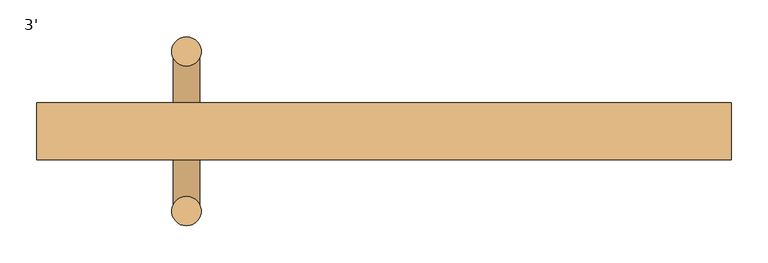
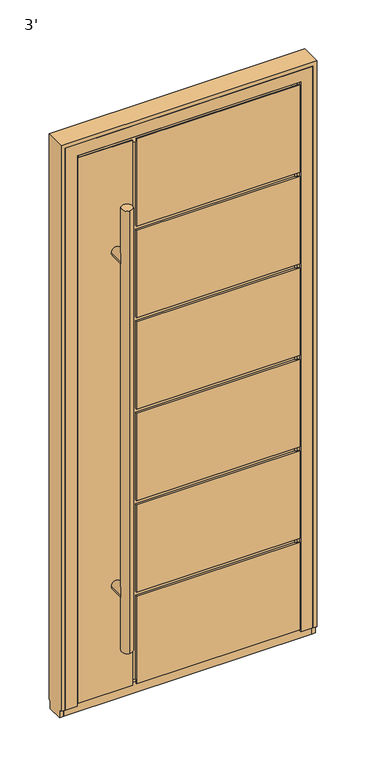
"""IFC4 building model written with IfcOpenShell, lengths in millimetres: door geometry, 3'."""

from ifc_helpers import new_model, si_unit, point, frame, frame_2d, origin, place, context, project, spatial, circle_curve, trimmed, segment, composite_curve, outline, extrude, faceted_brep, source, transform, mapped, element, save


def door_3_79df91aa(model_context):
    return source(origin(), model_context, "Body", "SolidModel", [
        extrude(outline(composite_curve([segment(trimmed(circle_curve(frame_2d((-268.65, 90.8003001)), 20.0), [point((-268.65, 70.8003001))], [point((-268.65, 110.8003001))], False, "CARTESIAN"), True, "CONTINUOUS"), segment(trimmed(circle_curve(frame_2d((-268.65, 90.8003001)), 20.0), [point((-268.65, 110.8003001))], [point((-268.65, 70.8003001))], False, "CARTESIAN"), True, "CONTINUOUS")], self_intersect=False)), frame((0.0, 0.0, 210.0000003), z_axis=(0.0, 0.0, 1.0), x_axis=(1.0, 0.0, 0.0)), (0.0, 0.0, 1.0), 1724.5),
        extrude(outline(composite_curve([segment(trimmed(circle_curve(frame_2d((-268.65, -126.2003001)), 20.0), [point((-268.65, -146.2003001))], [point((-268.65, -106.2003001))], False, "CARTESIAN"), True, "CONTINUOUS"), segment(trimmed(circle_curve(frame_2d((-268.65, -126.2003001)), 20.0), [point((-268.65, -106.2003001))], [point((-268.65, -146.2003001))], False, "CARTESIAN"), True, "CONTINUOUS")], self_intersect=False)), frame((0.0, 0.0, 210.0000003), z_axis=(0.0, 0.0, 1.0), x_axis=(1.0, 0.0, 0.0)), (0.0, 0.0, 1.0), 1724.5),
        extrude(outline(composite_curve([segment(trimmed(circle_curve(frame_2d((422.2500003, -268.65)), 18.0), [point((422.2500003, -286.65))], [point((422.2500003, -250.65))], False, "CARTESIAN"), True, "CONTINUOUS"), segment(trimmed(circle_curve(frame_2d((422.2500003, -268.65)), 18.0), [point((422.2500003, -250.65))], [point((422.2500003, -286.65))], False, "CARTESIAN"), True, "CONTINUOUS")], self_intersect=False)), frame((0.0, -126.2, 0.0), z_axis=(0.0, 1.0, 0.0), x_axis=(0.0, 0.0, 1.0)), (0.0, 0.0, 1.0), 217.0),
        extrude(outline(composite_curve([segment(trimmed(circle_curve(frame_2d((1722.2500003, -268.65)), 18.0), [point((1722.2500003, -286.65))], [point((1722.2500003, -250.65))], False, "CARTESIAN"), True, "CONTINUOUS"), segment(trimmed(circle_curve(frame_2d((1722.2500003, -268.65)), 18.0), [point((1722.2500003, -250.65))], [point((1722.2500003, -286.65))], False, "CARTESIAN"), True, "CONTINUOUS")], self_intersect=False)), frame((0.0, -126.2, 0.0), z_axis=(0.0, 1.0, 0.0), x_axis=(0.0, 0.0, 1.0)), (0.0, 0.0, 1.0), 217.0),
        faceted_brep([(-193.65, 13.8, 366.5833337), (383.65, 13.8, 366.5833337), (383.65, 13.8, 351.5833337), (-193.65, 13.8, 351.5833337), (-193.65, 13.8, 35.0), (-208.65, 13.8, 35.0), (-208.65, 13.8, 2109.5000003), (-193.65, 13.8, 2109.5000003), (-193.65, 13.8, 1792.916667), (383.65, 13.8, 1792.916667), (383.65, 13.8, 1777.916667), (-193.65, 13.8, 1777.916667), (-193.65, 13.8, 1436.3333337), (383.65, 13.8, 1436.3333337), (383.65, 13.8, 1421.3333337), (-193.65, 13.8, 1421.3333337), (-193.65, 13.8, 1079.7500004), (383.65, 13.8, 1079.7500004), (383.65, 13.8, 1064.7500004), (-193.65, 13.8, 1064.7500004), (-193.65, 13.8, 723.166667), (383.65, 13.8, 723.166667), (383.65, 13.8, 708.166667), (-193.65, 13.8, 708.166667), (-193.65, 20.8, 708.166667), (-193.65, 20.8, 366.5833337), (383.65, 20.8, 708.166667), (383.65, 11.7997698, 2109.5000003), (383.65, 11.7997698, 35.0), (383.65, 18.8020472, 35.0), (383.65, 18.8020472, 24.0), (383.65, 20.8, 24.0), (383.65, 20.8, 351.5833337), (383.65, 20.8, 366.5833337), (383.65, 20.8, 723.166667), (383.65, 20.8, 1064.7500004), (383.65, 20.8, 1079.7500004), (383.65, 20.8, 1421.3333337), (383.65, 20.8, 1436.3333337), (383.65, 20.8, 1777.916667), (383.65, 20.8, 1792.916667), (383.65, 20.8, 2109.5000003), (-193.65, 20.8, 723.166667), (-193.65, 20.8, 1064.7500004), (-193.65, 20.8, 1079.7500004), (-193.65, 20.8, 1421.3333337), (-208.65, 18.8020472, 35.0), (-208.65, 18.8020472, 24.0), (-208.65, 20.8, 24.0), (-208.65, 20.8, 2109.5000003), (-383.65, 11.7997698, 35.0), (-383.65, 18.8020472, 35.0), (-193.65, 18.8020472, 35.0), (-193.65, 20.8, 351.5833337), (-193.65, 20.8, 24.0), (-193.65, 18.8020472, 24.0), (-383.65, 18.8020472, 24.0), (-383.65, 20.8, 24.0), (-383.65, 20.8, 2109.5000003), (-193.65, 20.8, 1436.3333337), (-193.65, 20.8, 1777.916667), (-193.65, 20.8, 1792.916667), (-193.65, 20.8, 2109.5000003), (408.65, -56.2, 10.0000003), (-193.65, -56.2, 10.0000003), (-193.65, -53.2, 10.0000003), (408.65, -53.2, 10.0000003), (-408.65, -53.2, 10.0000003), (-208.65, -53.2, 10.0000003), (-208.65, -56.2, 10.0000003), (-408.65, -56.2, 10.0000003), (408.65, -56.2, 366.5833337), (408.65, -53.2, 366.5833337), (408.65, -53.2, 708.166667), (408.65, -56.2, 708.166667), (408.65, -56.2, 1079.7500004), (408.65, -53.2, 1079.7500004), (408.65, -53.2, 1421.3333337), (408.65, -56.2, 1421.3333337), (408.65, -56.2, 723.166667), (408.65, -53.2, 723.166667), (408.65, -53.2, 1064.7500004), (408.65, -56.2, 1064.7500004), (408.65, -56.2, 1436.3333337), (408.65, -53.2, 1436.3333337), (408.65, -53.2, 1777.916667), (408.65, -56.2, 1777.916667), (408.65, -56.2, 2134.5000003), (408.65, -56.2, 1792.916667), (408.65, -53.2, 1792.916667), (408.65, -53.2, 2134.5000003), (408.65, -53.2, 351.5833337), (408.65, -56.2, 351.5833337), (-193.65, -53.2, 25.5), (393.15, -53.2, 25.5), (393.15, -53.2, 351.5833337), (393.15, -53.2, 366.5833337), (393.15, -53.2, 708.166667), (393.15, -53.2, 1079.7500004), (393.15, -53.2, 1421.3333337), (393.15, -53.2, 723.166667), (393.15, -53.2, 1064.7500004), (-393.15, -53.2, 25.5), (-208.65, -53.2, 25.5), (-408.65, -53.2, 2134.5000003), (-208.65, -53.2, 2134.5000003), (-208.65, -53.2, 2119.0000003), (-393.15, -53.2, 2119.0000003), (393.15, -53.2, 1436.3333337), (393.15, -53.2, 1777.916667), (393.15, -53.2, 1792.916667), (393.15, -53.2, 2119.0000003), (-193.65, -53.2, 2119.0000003), (-193.65, -53.2, 2134.5000003), (-193.65, -49.2, 351.5833337), (-193.65, -49.2, 25.5), (-193.65, -56.2, 351.5833337), (-208.65, -56.2, 2134.5000003), (-408.65, -56.2, 2134.5000003), (-193.65, -56.2, 708.166667), (-193.65, -56.2, 366.5833337), (-193.65, -56.2, 1421.3333337), (-193.65, -56.2, 1079.7500004), (-193.65, -56.2, 1064.7500004), (-193.65, -56.2, 723.166667), (-193.65, -56.2, 1777.916667), (-193.65, -56.2, 1436.3333337), (-193.65, -56.2, 2134.5000003), (-193.65, -56.2, 1792.916667), (-208.65, -49.2, 2119.0000003), (-208.65, -49.2, 25.5), (-383.65, 11.7997698, 2109.5000003), (393.15, 11.7997698, 2119.0000003), (393.15, 11.7997698, 25.5), (-393.15, 11.7997698, 25.5), (-393.15, 11.7997698, 2119.0000003), (393.15, -49.2, 1792.916667), (393.15, -49.2, 1777.916667), (393.15, -49.2, 1436.3333337), (393.15, -49.2, 1421.3333337), (393.15, -49.2, 1079.7500004), (393.15, -49.2, 1064.7500004), (393.15, -49.2, 723.166667), (393.15, -49.2, 708.166667), (393.15, -49.2, 366.5833337), (393.15, -49.2, 351.5833337), (-193.65, -49.2, 1777.916667), (-193.65, -49.2, 1792.916667), (-193.65, -49.2, 2119.0000003), (-193.65, -49.2, 366.5833337), (-193.65, -49.2, 708.166667), (-193.65, -49.2, 723.166667), (-193.65, -49.2, 1064.7500004), (-193.65, -49.2, 1079.7500004), (-193.65, -49.2, 1421.3333337), (-193.65, -49.2, 1436.3333337)], [[[0, 1, 2, 3, 4, 5, 6, 7, 8, 9, 10, 11, 12, 13, 14, 15, 16, 17, 18, 19, 20, 21, 22, 23]], [[23, 24, 25, 0]], [[23, 22, 26, 24]], [[27, 28, 29, 30, 31, 32, 2, 1, 33, 26, 22, 21, 34, 35, 18, 17, 36, 37, 14, 13, 38, 39, 10, 9, 40, 41]], [[42, 34, 21, 20]], [[19, 43, 42, 20]], [[19, 18, 35, 43]], [[44, 36, 17, 16]], [[15, 45, 44, 16]], [[5, 46, 47, 48, 49, 6]], [[28, 50, 51, 46, 5, 4, 52, 29]], [[53, 54, 55, 52, 4, 3]], [[3, 2, 32, 53]], [[25, 33, 1, 0]], [[29, 52, 55, 30]], [[56, 47, 46, 51]], [[30, 55, 54, 31]], [[57, 48, 47, 56]], [[36, 44, 45, 37]], [[34, 42, 43, 35]], [[33, 25, 24, 26]], [[54, 53, 32, 31]], [[58, 49, 48, 57]], [[38, 59, 60, 39]], [[41, 40, 61, 62]], [[63, 64, 65, 66]], [[67, 68, 69, 70]], [[71, 72, 73, 74]], [[75, 76, 77, 78]], [[79, 80, 81, 82]], [[83, 84, 85, 86]], [[87, 88, 89, 90]], [[66, 91, 92, 63]], [[65, 93, 94, 95, 91, 66]], [[72, 96, 97, 73]], [[76, 98, 99, 77]], [[80, 100, 101, 81]], [[102, 103, 68, 67, 104, 105, 106, 107]], [[84, 108, 109, 85]], [[90, 89, 110, 111, 112, 113]], [[114, 115, 93, 65, 64, 116]], [[70, 69, 117, 118]], [[63, 92, 116, 64]], [[74, 119, 120, 71]], [[78, 121, 122, 75]], [[82, 123, 124, 79]], [[86, 125, 126, 83]], [[87, 127, 128, 88]], [[70, 118, 104, 67]], [[129, 106, 105, 117, 69, 68, 103, 130]], [[58, 57, 56, 51, 50, 131]], [[132, 133, 134, 135], [131, 50, 28, 27]], [[111, 110, 136, 137, 109, 108, 138, 139, 99, 98, 140, 141, 101, 100, 142, 143, 97, 96, 144, 145, 95, 94, 133, 132]], [[94, 93, 115, 130, 103, 102, 134, 133]], [[135, 134, 102, 107]], [[146, 137, 136, 147, 148, 129, 130, 115, 114, 145, 144, 149, 150, 143, 142, 151, 152, 141, 140, 153, 154, 139, 138, 155]], [[153, 122, 121, 154]], [[153, 140, 98, 76, 75, 122]], [[123, 82, 81, 101, 141, 152]], [[151, 124, 123, 152]], [[151, 142, 100, 80, 79, 124]], [[119, 74, 73, 97, 143, 150]], [[149, 120, 119, 150]], [[149, 144, 96, 72, 71, 120]], [[116, 92, 91, 95, 145, 114]], [[15, 14, 37, 45]], [[59, 38, 13, 12]], [[11, 60, 59, 12]], [[11, 10, 39, 60]], [[61, 40, 9, 8]], [[8, 7, 62, 61]], [[125, 86, 85, 109, 137, 146]], [[128, 127, 113, 112, 148, 147]], [[121, 78, 77, 99, 139, 154]], [[155, 138, 108, 84, 83, 126]], [[155, 126, 125, 146]], [[147, 136, 110, 89, 88, 128]], [[90, 113, 127, 87]], [[118, 117, 105, 104]], [[132, 135, 107, 106, 129, 148, 112, 111]], [[27, 41, 62, 7, 6, 49, 58, 131]]]),
        faceted_brep([(-457.2, -56.2, 0.0), (-457.2, -47.1997571, 0.0), (-412.7, -47.1997571, 0.0), (-412.7, -56.2, 0.0), (-403.2, 16.2999958, 0.0), (-403.2, 11.8, 0.0), (-457.2, 11.8, 0.0), (-457.2, 20.8, 0.0), (-387.7, 20.8, 0.0), (-387.7, 16.2999958, 0.0), (457.2, 20.8, 0.0), (457.2, 11.8, 0.0), (403.2, 11.8, 0.0), (403.2, 16.2999958, 0.0), (387.7, 16.2999958, 0.0), (387.7, 20.8, 0.0), (412.7, -47.1997571, 0.0), (457.2, -47.1997571, 0.0), (457.2, -56.2, 0.0), (412.7, -56.2, 0.0), (-457.2, 11.8, -30.0), (-457.2, -47.1997571, -30.0), (-457.2, -56.2, 2189.5), (-457.2, 20.8, 2189.5), (-412.7, -56.2, 2145.0), (412.7, -56.2, 2145.0), (457.2, -56.2, 2189.5), (457.2, 20.8, 2189.5), (457.2, -47.1997571, -30.0), (457.2, 11.8, -30.0), (387.7, 20.8, 2120.0), (-387.7, 20.8, 2120.0), (-403.2, -47.2, 2135.5), (-403.2, -47.2, 14.5), (-403.2, 11.8, 14.5), (-403.2, 16.2999958, 2135.5), (403.2, 16.2999958, 2135.5), (403.2, -47.2, 2135.5), (403.2, 11.8, 14.5), (403.2, -47.2, 14.5), (-412.7, -47.2, 2145.0), (412.7, -47.2, 2145.0), (-387.7, 16.2999958, 2120.0), (387.7, 16.2999958, 2120.0)], [[[0, 1, 2, 3]], [[4, 5, 6, 7, 8, 9]], [[10, 11, 12, 13, 14, 15]], [[16, 17, 18, 19]], [[7, 6, 20, 21, 1, 0, 22, 23]], [[3, 24, 25, 19, 18, 26, 22, 0]], [[22, 26, 27, 23]], [[18, 17, 28, 29, 11, 10, 27, 26]], [[7, 23, 27, 10, 15, 30, 31, 8]], [[32, 33, 34, 5, 4, 35]], [[35, 36, 37, 32]], [[36, 13, 12, 38, 39, 37]], [[40, 24, 3, 2]], [[16, 41, 40, 2, 1, 21, 28, 17], [37, 39, 33, 32]], [[9, 42, 43, 14, 13, 36, 35, 4]], [[8, 31, 42, 9]], [[24, 40, 41, 25]], [[30, 43, 42, 31]], [[19, 25, 41, 16]], [[14, 43, 30, 15]], [[20, 6, 5, 34, 38, 12, 11, 29]], [[39, 38, 34, 33]], [[20, 29, 28, 21]]]),
        faceted_brep([(-457.2, -47.2, -30.0), (-472.2, -47.2, -30.0), (-472.2, 11.8, -30.0), (-457.2, 11.8, -30.0), (-457.2, -56.2, 2189.5), (-457.2, -56.2, 0.0), (-457.2, -47.2, 0.0), (-457.2, 11.8, 0.0), (-457.2, 20.8, 0.0), (-457.2, 20.8, 2189.5), (-472.2, 11.8, 0.0), (472.2, 11.8, 0.0), (472.2, 11.8, -30.0), (457.2, 11.8, -30.0), (457.2, 11.8, 0.0), (-472.2, 20.8, 2204.5), (-472.2, 20.8, 0.0), (-472.2, -47.2, 0.0), (-472.2, -56.2, 0.0), (-472.2, -56.2, 2204.5), (457.2, -47.2, 0.0), (457.2, -47.2, -30.0), (472.2, -47.2, -30.0), (472.2, -47.2, 0.0), (457.2, 20.8, 2189.5), (457.2, 20.8, 0.0), (457.2, -56.2, 0.0), (457.2, -56.2, 2189.5), (472.2, -56.2, 0.0), (472.2, -56.2, 2204.5), (472.2, 20.8, 0.0), (472.2, 20.8, 2204.5)], [[[0, 1, 2, 3]], [[4, 5, 6, 0, 3, 7, 8, 9]], [[7, 3, 2, 10]], [[11, 12, 13, 14]], [[15, 16, 10, 2, 1, 17, 18, 19]], [[17, 1, 0, 6]], [[20, 21, 22, 23]], [[24, 25, 14, 13, 21, 20, 26, 27]], [[27, 26, 28, 29, 19, 18, 5, 4]], [[6, 5, 18, 17]], [[23, 28, 26, 20]], [[22, 21, 13, 12]], [[10, 16, 8, 7]], [[14, 25, 30, 11]], [[9, 8, 16, 15, 31, 30, 25, 24]], [[29, 28, 23, 22, 12, 11, 30, 31]], [[9, 24, 27, 4]], [[19, 29, 31, 15]]]),
    ])


if __name__ == "__main__":
    model = new_model("IFC4")
    model_context = context("Model", 3, world=origin())
    ifc_project = project(units=[si_unit("LENGTHUNIT", "METRE", prefix="MILLI")], contexts=[model_context])
    site = spatial("IfcSite", under=ifc_project)
    building = spatial("IfcBuilding", under=site)
    placement = place(None, origin())
    door_3_shape = door_3_79df91aa(model_context)
    element("IfcDoor", 1, ObjectType="3'", at=placement, inside=building, context=model_context, shape_type="MappedRepresentation", body=[
        mapped(door_3_shape, transform((0.0, 0.0, 0.0), x_axis=(1.0, 0.0, 0.0), y_axis=(0.0, 1.0, 0.0), z_axis=(0.0, 0.0, 1.0))),
    ])
    save(model, "model.ifc")

# Revit data of these elements
# Type "3'"
#   Type Mark = "10"
#   Water resistance = "up to Class E900, EN 12208:2001"
#   Uniclass2015Version = "v1.21"
#   Uniclass2015Reference = "Ss_25_30_20_30"
#   Uniclass2015Description = "Frame and door leaf system"
#   URL = "www.aluprof.com"
#   Type IFC Predefined Type = "USERDEFINED"
#   Right-hand / Left-hand door [instance default] = ""
#   Resistance to wind load = "up to Class C5/B5, EN 12210:2001"
#   Insert type = "ST"
#   Hardware [instance default] = ""
#   Product page = "https://aluprof.com/en/architects/offer/window-and-door-systems/panel-doors#visualisation"
#   Operation = "SinglePanelOutwardOpening"
#   Opening type = "Outward"
#   NBSReference = "25-50-20/125"
#   NBSDescription = "Frame and door leaf system"
#   Important = "The actual acceptable construction dimensions are dependent on the selection of profiles and hardware, glazing type, construction weight and the construction’s operating conditions. These should be determined by a suitably qualified person, and using ALUPROF’s calculation software"
#   IfcExportType = "USERDEFINED"
#   IfcExportAs = "IfcDoorType"
#   Handle type [instance default] = ""
#   Manufacturer = "ALUPROF SA"
#   Export Type to IFC As = "IfcDoorType"
#   Door sill type [instance default] = ""
#   Description = "External single-leaf panel door outward opening"
#   Model = "MB-86 ST Panel Door AD07"
#   Content of the recyclate in the material = "69.2%"
#   COBie.Type.WarrantyDurationParts = ""
#   COBie.Type.Name = ""
#   COBie.Type.Manufacturer = "ALUPROF SA"
#   COBie.Space.Name = ""
#   COBie.Floor.Name = ""
#   COBie.Facility.Name = ""
#   COBie.CreatedOn = ""
#   COBie.Component.WarrantyStartDate = ""
#   COBie.Component.Name = "MB-86 ST Panel Door AD07"
#   Burglar resistance = "RC2"
#   Air permeability = "up to Class 4, EN 12207:2001"
#   Width of the active leaf = 2' - 8.17717"
#   Placement in wall = 0' - 0.7874"
#   Thickness = 0' - 3.0315"
#   Height of the opening sash = 6' - 11.64173"
#   Handle Offset = 3' - 5.33858"
#   Rough Height = 7' - 4.61024"
#   Rough Width = 3' - 1.1811"
#   Height = 7' - 2.20079"
#   Width = 3' - 0"
#   Construction depth = 0' - 3.0315"
#   Clear opening width = 2' - 3.94882"
#   Clear opening height = 6' - 10.67717"
#   Height of the array = 1' - 1.44816"
#   Schedule No. [instance default] = 1
#   Handrail [instance default] = yes
#   IsExternal = yes
#   Handle [instance default] = no
#   Door closer [instance default] = no
#   Function = 1
#   COBie.Type = yes
#   COBie = yes
#   Access control [instance default] = no
#   Panel = element 346771
#   Wall Closure = (empty or 0)
